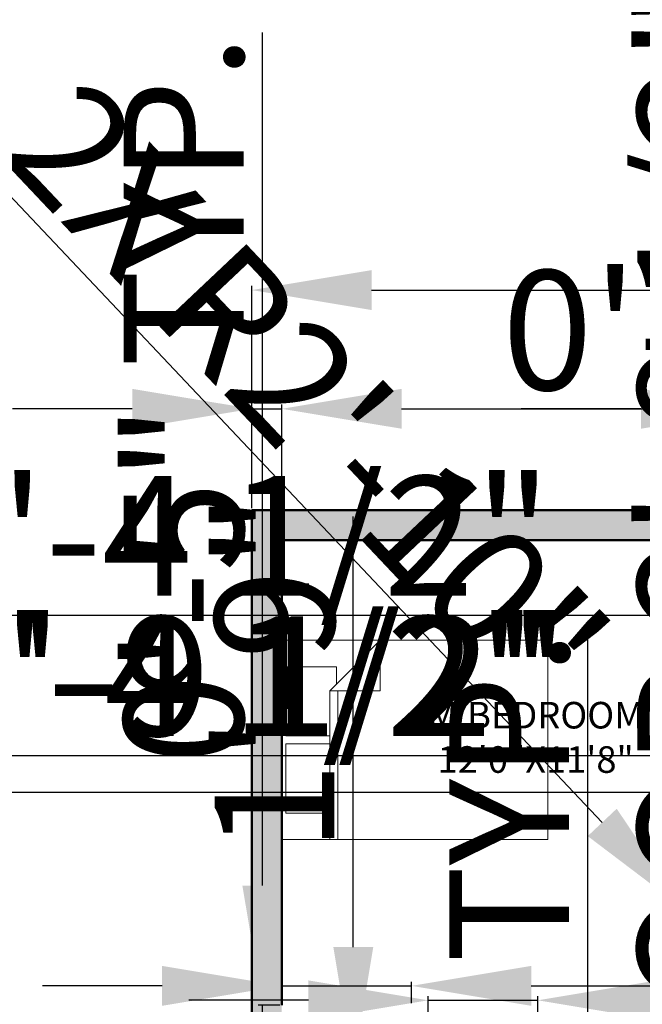
# Model space of a CAD drawing. Units: inches. Extents: x -299 to 1164, y -2 to 940.
# Tile 7 of 11: x 189 to 376, y 490 to 786. Entities that reach past the tile are written whole.
import ezdxf

# ---------------------------------------------------------------- set-up
doc = ezdxf.new("R2010")
doc.units = ezdxf.units.IN
for name, color, linetype, lineweight in [('A-AREA-IDEN', 3, 'Continuous', 25), ('A-FURN', 8, 'Continuous', 18), ('dimensions', 191, 'Continuous', 18), ('outer walls', 7, 'Continuous', 50)]:
    doc.layers.add(name, color=color, linetype=linetype, lineweight=lineweight)
doc.layers.add('A-WALL-PATT', color=240, linetype='Continuous', lineweight=13, true_color=0xed1f24)
doc.styles.get("Standard").update_dxf_attribs({"font": 'arial.ttf'})
doc.dimstyles.new('ISO-25', dxfattribs={"dimtxt": 36, "dimasz": 36, "dimexe": 1.25, "dimexo": 0.625, "dimtad": 1, "dimlunit": 3, "dimtxsty": 'Standard', "dimcen": 2.5, "dimazin": 0, "dimtfac": 1, "dimtmove": 0, "dimatfit": 3, "dimfxl": 1, "dimarcsym": 0})

# ---------------------------------------------------------------- blocks, each defined once
blk = doc.blocks.new('Bed - Queen')
for p, q in [((0, -80.00003), (0, 0)), ((0, 0), (59.99999, 0)), ((59.99999, 0), (59.99999, -80.00003)), ((7.99999, -1.2), (28.79998, -1.2)), ((7.99999, -14.4), (7.99999, -1.2)), ((28.79998, -1.2), (28.79998, -14.4)), ((31.19999, -1.2), (51.99999, -1.2)), ((31.19999, -14.4), (31.19999, -1.2)), ((51.99999, -1.2), (51.99999, -16.4)), ((0, -14.4), (44.8, -14.4)), ((59.99999, -29.6), (44.8, -14.4)), ((44.8, -14.4), (44.8, -29.6)), ((44.8, -16.8), (0, -16.8)), ((51.99999, -16.4), (46.79936, -16.4)), ((44.8, -29.6), (59.99999, -29.6)), ((59.99999, -80.00003), (0, -80.00003))]:
    blk.add_line(p, q)
blk = doc.blocks.new('*D13')
at = {"layer": 'Defpoints', "color": 0, "transparency": 16777216}
for p in [(739.07, 704.71), (259.07, 638.49), (739.07, 638.49)]:
    blk.add_point(p, dxfattribs=at)
at = {"layer": 'dimensions', "color": 0, "lineweight": -2, "transparency": 16777216}
for p, q in [((259.07, 639.11), (259.07, 705.96)), ((739.07, 639.11), (739.07, 705.96)), ((295.07, 704.71), (703.07, 704.71))]:
    blk.add_line(p, q, dxfattribs=at)
at = {"layer": 'dimensions', "color": 0, "transparency": 16777216}
for points in [[(295.07, 710.71), (295.07, 698.71), (259.07, 704.71)], [(703.07, 710.71), (703.07, 698.71), (739.07, 704.71)]]:
    blk.add_solid(points, dxfattribs=at)
at = {"layer": 'dimensions', "color": 0, "transparency": 16777216, "insert": (499.07, 723.71), "char_height": 36, "attachment_point": 5}
blk.add_mtext("40'", dxfattribs=at)
blk = doc.blocks.new('*D26')
at = {"layer": 'Defpoints', "color": 0, "transparency": 16777216}
for p in [(415.32, 606.83), (415.32, 597.1), (443.65, 597.1)]:
    blk.add_point(p, dxfattribs=at)
at = {"layer": 'dimensions', "color": 0, "lineweight": -2, "transparency": 16777216}
for p, q in [((415.32, 597.72), (415.32, 608.08)), ((443.65, 597.72), (443.65, 608.08)), ((379.32, 606.83), (161.88, 606.83)), ((443.65, 606.83), (415.32, 606.83)), ((479.65, 606.83), (515.65, 606.83))]:
    blk.add_line(p, q, dxfattribs=at)
at = {"layer": 'dimensions', "color": 0, "transparency": 16777216}
for points in [[(379.32, 612.83), (379.32, 600.83), (415.32, 606.83)], [(479.65, 612.83), (479.65, 600.83), (443.65, 606.83)]]:
    blk.add_solid(points, dxfattribs=at)
at = {"layer": 'dimensions', "color": 0, "transparency": 16777216, "insert": (252.6, 626.07), "char_height": 36, "attachment_point": 5}
blk.add_mtext('2\'-4 1/2"', dxfattribs=at)
blk = doc.blocks.new('*D27')
at = {"layer": 'Defpoints', "color": 0, "transparency": 16777216}
for p in [(412.07, 375.49), (416.95, 375.49), (412.07, 342.99)]:
    blk.add_point(p, dxfattribs=at)
at = {"layer": 'dimensions', "color": 0, "lineweight": -2, "transparency": 16777216}
for p, q in [((416.95, 411.49), (416.95, 915.12)), ((412.7, 375.49), (418.2, 375.49)), ((416.95, 342.99), (416.95, 375.49)), ((412.7, 342.99), (418.2, 342.99)), ((416.95, 306.99), (416.95, 270.99))]:
    blk.add_line(p, q, dxfattribs=at)
at = {"layer": 'dimensions', "color": 0, "transparency": 16777216}
for points in [[(410.95, 411.49), (422.95, 411.49), (416.95, 375.49)], [(410.95, 306.99), (422.95, 306.99), (416.95, 342.99)]]:
    blk.add_solid(points, dxfattribs=at)
at = {"layer": 'dimensions', "color": 0, "transparency": 16777216, "insert": (397.69, 681.3), "char_height": 36, "attachment_point": 5, "rotation": 90}
blk.add_mtext('DOOR 2\'-8 1/2" TYP.', dxfattribs=at)
blk = doc.blocks.new('*D32')
at = {"layer": 'Defpoints', "color": 0, "transparency": 16777216}
for p in [(348.07, 310.2), (360.07, 310.2), (348.07, 250.2)]:
    blk.add_point(p, dxfattribs=at)
at = {"layer": 'dimensions', "color": 0, "lineweight": -2, "transparency": 16777216}
for p, q in [((360.07, 346.2), (360.07, 602.89)), ((348.7, 310.2), (361.32, 310.2)), ((360.07, 250.2), (360.07, 310.2)), ((348.7, 250.2), (361.32, 250.2)), ((360.07, 214.2), (360.07, 178.2))]:
    blk.add_line(p, q, dxfattribs=at)
at = {"layer": 'dimensions', "color": 0, "transparency": 16777216}
for points in [[(354.07, 346.2), (366.07, 346.2), (360.07, 310.2)], [(354.07, 214.2), (366.07, 214.2), (360.07, 250.2)]]:
    blk.add_solid(points, dxfattribs=at)
at = {"layer": 'dimensions', "color": 0, "transparency": 16777216, "insert": (341.07, 492.55), "char_height": 36, "attachment_point": 5, "rotation": 90}
blk.add_mtext('5\'-0" TYP.', dxfattribs=at)
blk = doc.blocks.new('*D34')
at = {"layer": 'Defpoints', "color": 0, "transparency": 16777216}
for p in [(443.84, 222.49), (447.44, 222.49), (443.84, 213.49)]:
    blk.add_point(p, dxfattribs=at)
at = {"layer": 'dimensions', "color": 0, "lineweight": -2, "transparency": 16777216}
for p, q in [((447.44, 258.49), (447.44, 515.18)), ((444.47, 222.49), (448.69, 222.49)), ((447.44, 213.49), (447.44, 222.49)), ((444.47, 213.49), (448.69, 213.49)), ((447.44, 177.49), (447.44, 141.49))]:
    blk.add_line(p, q, dxfattribs=at)
at = {"layer": 'dimensions', "color": 0, "transparency": 16777216}
for points in [[(441.44, 258.49), (453.44, 258.49), (447.44, 222.49)], [(441.44, 177.49), (453.44, 177.49), (447.44, 213.49)]]:
    blk.add_solid(points, dxfattribs=at)
at = {"layer": 'dimensions', "color": 0, "transparency": 16777216, "insert": (428.44, 404.83), "char_height": 36, "attachment_point": 5, "rotation": 90}
blk.add_mtext('0\'-9" TYP.', dxfattribs=at)
blk = doc.blocks.new('*D35')
at = {"layer": 'Defpoints', "color": 0, "transparency": 16777216}
for p in [(307.07, 495.34), (268.07, 489.49), (307.07, 489.49)]:
    blk.add_point(p, dxfattribs=at)
at = {"layer": 'dimensions', "color": 0, "lineweight": -2, "transparency": 16777216}
for p, q in [((232.07, 495.34), (196.07, 495.34)), ((268.07, 490.11), (268.07, 496.59)), ((268.07, 495.34), (307.07, 495.34)), ((307.07, 490.11), (307.07, 496.59)), ((343.07, 495.34), (749.73, 495.34))]:
    blk.add_line(p, q, dxfattribs=at)
at = {"layer": 'dimensions', "color": 0, "transparency": 16777216}
for points in [[(232.07, 501.34), (232.07, 489.34), (268.07, 495.34)], [(343.07, 501.34), (343.07, 489.34), (307.07, 495.34)]]:
    blk.add_solid(points, dxfattribs=at)
at = {"layer": 'dimensions', "color": 0, "transparency": 16777216, "insert": (564.4, 514.36), "char_height": 36, "attachment_point": 5}
blk.add_mtext('VENT 3\'-3" TYP.', dxfattribs=at)
blk = doc.blocks.new('*D36')
at = {"layer": 'Defpoints', "color": 0, "transparency": 16777216}
for p in [(262.22, 489.49), (268.07, 489.49), (268.07, 484.49)]:
    blk.add_point(p, dxfattribs=at)
at = {"layer": 'dimensions', "color": 0, "lineweight": -2, "transparency": 16777216}
for p, q in [((262.22, 525.49), (262.22, 782.18)), ((267.45, 489.49), (260.97, 489.49)), ((262.22, 484.49), (262.22, 489.49)), ((267.45, 484.49), (260.97, 484.49)), ((262.22, 448.49), (262.22, 412.49))]:
    blk.add_line(p, q, dxfattribs=at)
at = {"layer": 'dimensions', "color": 0, "transparency": 16777216}
for points in [[(256.22, 525.49), (268.22, 525.49), (262.22, 489.49)], [(256.22, 448.49), (268.22, 448.49), (262.22, 484.49)]]:
    blk.add_solid(points, dxfattribs=at)
at = {"layer": 'dimensions', "color": 0, "transparency": 16777216, "insert": (243.22, 671.83), "char_height": 36, "attachment_point": 5, "rotation": 90}
blk.add_mtext('0\'-5" TYP.', dxfattribs=at)
blk = doc.blocks.new('*D43')
at = {"layer": 'Defpoints', "color": 0, "transparency": 16777216}
for p in [(268.07, 668.99), (259.07, 638.49), (268.07, 629.49)]:
    blk.add_point(p, dxfattribs=at)
at = {"layer": 'dimensions', "color": 0, "lineweight": -2, "transparency": 16777216}
for p, q in [((259.07, 639.11), (259.07, 670.24)), ((268.07, 630.11), (268.07, 670.24)), ((223.07, 668.99), (187.07, 668.99)), ((259.07, 668.99), (268.07, 668.99)), ((304.07, 668.99), (437.02, 668.99))]:
    blk.add_line(p, q, dxfattribs=at)
at = {"layer": 'dimensions', "color": 0, "transparency": 16777216}
for points in [[(223.07, 674.99), (223.07, 662.99), (259.07, 668.99)], [(304.07, 674.99), (304.07, 662.99), (268.07, 668.99)]]:
    blk.add_solid(points, dxfattribs=at)
at = {"layer": 'dimensions', "color": 0, "transparency": 16777216, "insert": (388.54, 687.99), "char_height": 36, "attachment_point": 5}
blk.add_mtext('0\'-9"', dxfattribs=at)
blk = doc.blocks.new('*D44')
at = {"layer": 'Defpoints', "color": 0, "transparency": 16777216}
for p in [(417.07, 668.99), (412.07, 629.49), (417.07, 629.49)]:
    blk.add_point(p, dxfattribs=at)
at = {"layer": 'dimensions', "color": 0, "lineweight": -2, "transparency": 16777216}
for p, q in [((412.07, 630.11), (412.07, 670.24)), ((417.07, 630.11), (417.07, 670.24)), ((376.07, 668.99), (340.07, 668.99)), ((412.07, 668.99), (417.07, 668.99)), ((453.07, 668.99), (586.02, 668.99))]:
    blk.add_line(p, q, dxfattribs=at)
at = {"layer": 'dimensions', "color": 0, "transparency": 16777216}
for points in [[(376.07, 674.99), (376.07, 662.99), (412.07, 668.99)], [(453.07, 674.99), (453.07, 662.99), (417.07, 668.99)]]:
    blk.add_solid(points, dxfattribs=at)
at = {"layer": 'dimensions', "color": 0, "transparency": 16777216, "insert": (537.54, 687.99), "char_height": 36, "attachment_point": 5}
blk.add_mtext('0\'-5"', dxfattribs=at)
blk = doc.blocks.new('*D53')
at = {"layer": 'Defpoints', "color": 0, "transparency": 16777216}
for p in [(177.57, 553.49), (586.07, 553.49), (586.07, 481.49)]:
    blk.add_point(p, dxfattribs=at)
at = {"layer": 'dimensions', "color": 0, "lineweight": -2, "transparency": 16777216}
for p, q in [((177.57, 589.49), (177.57, 722.63)), ((585.45, 553.49), (176.32, 553.49)), ((177.57, 481.49), (177.57, 553.49)), ((585.45, 481.49), (176.32, 481.49)), ((177.57, 445.49), (177.57, 409.49))]:
    blk.add_line(p, q, dxfattribs=at)
at = {"layer": 'dimensions', "color": 0, "transparency": 16777216}
for points in [[(171.57, 589.49), (183.57, 589.49), (177.57, 553.49)], [(171.57, 445.49), (183.57, 445.49), (177.57, 481.49)]]:
    blk.add_solid(points, dxfattribs=at)
at = {"layer": 'dimensions', "color": 0, "transparency": 16777216, "insert": (158.57, 674.06), "char_height": 36, "attachment_point": 5, "rotation": 90}
blk.add_mtext('6\'-0"', dxfattribs=at)
blk = doc.blocks.new('*D54')
at = {"layer": 'Defpoints', "color": 0, "transparency": 16777216}
for p in [(345.07, 490.99), (312.07, 460.49), (345.07, 460.49)]:
    blk.add_point(p, dxfattribs=at)
at = {"layer": 'dimensions', "color": 0, "lineweight": -2, "transparency": 16777216}
for p, q in [((312.07, 461.11), (312.07, 492.24)), ((345.07, 461.11), (345.07, 492.24)), ((276.07, 490.99), (240.07, 490.99)), ((312.07, 490.99), (345.07, 490.99)), ((381.07, 490.99), (514.63, 490.99))]:
    blk.add_line(p, q, dxfattribs=at)
at = {"layer": 'dimensions', "color": 0, "transparency": 16777216}
for points in [[(276.07, 496.99), (276.07, 484.99), (312.07, 490.99)], [(381.07, 496.99), (381.07, 484.99), (345.07, 490.99)]]:
    blk.add_solid(points, dxfattribs=at)
at = {"layer": 'dimensions', "color": 0, "transparency": 16777216, "insert": (465.85, 509.99), "char_height": 36, "attachment_point": 5}
blk.add_mtext('2\'-9"', dxfattribs=at)
blk = doc.blocks.new('*D55')
at = {"layer": 'Defpoints', "color": 0, "transparency": 16777216}
for p in [(289.57, 470.99), (320.07, 470.99), (320.07, 449.99)]:
    blk.add_point(p, dxfattribs=at)
at = {"layer": 'dimensions', "color": 0, "lineweight": -2, "transparency": 16777216}
for p, q in [((289.57, 506.99), (289.57, 636.55)), ((319.45, 470.99), (288.32, 470.99)), ((289.57, 449.99), (289.57, 470.99)), ((319.45, 449.99), (288.32, 449.99)), ((289.57, 413.99), (289.57, 377.99))]:
    blk.add_line(p, q, dxfattribs=at)
at = {"layer": 'dimensions', "color": 0, "transparency": 16777216}
for points in [[(283.57, 506.99), (295.57, 506.99), (289.57, 470.99)], [(283.57, 413.99), (295.57, 413.99), (289.57, 449.99)]]:
    blk.add_solid(points, dxfattribs=at)
at = {"layer": 'dimensions', "color": 0, "transparency": 16777216, "insert": (270.57, 589.77), "char_height": 36, "attachment_point": 5, "rotation": 90}
blk.add_mtext('1\'-9"', dxfattribs=at)
blk = doc.blocks.new('*D61')
at = {"layer": 'Defpoints', "color": 0, "transparency": 16777216}
for p in [(389.15, 518.35), (412.32, 493.81)]:
    blk.add_point(p, dxfattribs=at)
at = {"layer": 'dimensions', "color": 0, "lineweight": -2, "transparency": 16777216}
for p, q in [((176.74, 743.24), (364.43, 544.52)), ((412.32, 493.81), (389.15, 518.35))]:
    blk.add_line(p, q, dxfattribs=at)
at = {"layer": 'dimensions', "color": 0, "transparency": 16777216}
blk.add_solid([(368.79, 548.64), (360.07, 540.4), (389.15, 518.35)], dxfattribs=at)
at = {"layer": 'dimensions', "color": 0, "transparency": 16777216, "insert": (272.04, 670.02), "char_height": 36, "attachment_point": 5, "rotation": 313.3644}
blk.add_mtext('2X R2\'-10"', dxfattribs=at)
blk = doc.blocks.new('*D68')
at = {"layer": 'Defpoints', "color": 0, "transparency": 16777216}
for p in [(422.02, 564.66), (515.63, 564.66)]:
    blk.add_point(p, dxfattribs=at)
at = {"layer": 'dimensions', "color": 0, "lineweight": -2, "transparency": 16777216}
for p, q in [((134.73, 564.66), (386.02, 564.66)), ((515.63, 564.66), (422.02, 564.66))]:
    blk.add_line(p, q, dxfattribs=at)
at = {"layer": 'dimensions', "color": 0, "transparency": 16777216}
blk.add_solid([(386.02, 570.66), (386.02, 558.66), (422.02, 564.66)], dxfattribs=at)
at = {"layer": 'dimensions', "color": 0, "transparency": 16777216, "insert": (242.37, 583.9), "char_height": 36, "attachment_point": 5, "rotation": 359.9997}
blk.add_mtext('R7\'-9 1/2"', dxfattribs=at)
blk = doc.blocks.new('*D70')
at = {"layer": 'Defpoints', "color": 0, "transparency": 16777216}
for p in [(417.38, 564.66), (505.63, 564.66)]:
    blk.add_point(p, dxfattribs=at)
at = {"layer": 'dimensions', "color": 0, "lineweight": -2, "transparency": 16777216}
for p, q in [((130.1, 564.66), (381.38, 564.66)), ((505.63, 564.66), (417.38, 564.66))]:
    blk.add_line(p, q, dxfattribs=at)
at = {"layer": 'dimensions', "color": 0, "transparency": 16777216}
blk.add_solid([(381.38, 570.66), (381.38, 558.66), (417.38, 564.66)], dxfattribs=at)
at = {"layer": 'dimensions', "color": 0, "transparency": 16777216, "insert": (237.74, 583.9), "char_height": 36, "attachment_point": 5, "rotation": 359.9997}
blk.add_mtext('R7\'-4 1/2"', dxfattribs=at)

msp = doc.modelspace()

# ---------------------------------------------------------------- hatches: boundary and pattern name
at = {"layer": 'A-WALL-PATT'}
h = msp.add_hatch(color=256, dxfattribs=at)
h.dxf.hatch_style = 1
h.paths.add_polyline_path([(312.071, 460.489), (307.071, 460.489), (307.071, 432.489), (307.071, 427.489), (372.071, 427.489), (372.071, 375.489), (372.071, 370.489), (380.071, 370.489, -0.0217424), (380.071, 372.989), (380.071, 375.489), (377.071, 375.489), (377.071, 427.489), (417.071, 427.489), (417.071, 489.489), (412.071, 489.489), (412.071, 484.489), (412.071, 432.489), (312.071, 432.489)], flags=17)
h.paths.add_polyline_path([(340.071, 372.989, -0.0217424), (340.071, 375.489), (268.071, 375.489), (268.071, 427.489), (268.071, 432.489), (268.071, 484.489), (268.071, 489.489), (268.071, 629.489), (412.071, 629.489), (412.071, 527.563, -0.0185322), (414.571, 527.489), (417.071, 527.489), (417.071, 629.489), (581.071, 629.489), (581.071, 553.489), (586.071, 553.489), (586.071, 629.489), (730.071, 629.489), (730.071, 405.489), (713.071, 405.489), (713.071, 396.489), (739.071, 396.489), (739.071, 638.489), (259.071, 638.489), (259.071, 183.489), (304.071, 183.489), (304.071, 192.489), (268.071, 192.489), (268.071, 370.489), (340.071, 370.489)])
h.paths.add_polyline_path([(417.071, 188.489), (417.071, 213.489), (461.071, 213.489), (461.071, 188.489)], flags=16)
h.paths.add_polyline_path([(586.071, 313.578), (577.071, 313.578), (577.071, 311.489), (575.54, 311.489), (575.54, 302.489), (586.071, 302.489)], flags=16)
h.paths.add_polyline_path([(586.071, 405.489), (586.071, 481.489), (581.071, 481.489), (581.071, 432.489), (499.071, 432.489), (499.071, 427.489), (577.071, 427.489), (577.071, 385.578), (586.071, 385.578), (586.071, 396.489)], flags=17)
h.paths.add_polyline_path([(641.071, 405.489), (624.071, 405.489, -0.0333689), (624.071, 400.989), (624.071, 396.489), (641.071, 396.489)], flags=17)
h.paths.add_polyline_path([(491.866, 222.489), (491.866, 213.489), (586.071, 213.489), (586.071, 222.489)])
edge = h.paths.add_edge_path()
edge.add_line((467.866, 213.489), (467.866, 222.489))
edge.add_line((467.866, 222.489), (466.071, 222.489))
edge.add_line((466.071, 222.489), (466.071, 302.489))
edge.add_line((466.071, 302.489), (527.54, 302.489))
edge.add_line((527.54, 302.489), (527.54, 311.489))
edge.add_line((527.54, 311.489), (449.071, 311.489))
edge.add_line((449.071, 311.489), (449.071, 308.989))
edge.add_arc((420.339, 307.739), 28.759, -2.4911, 2.4911, ccw=False)
edge.add_line((449.071, 306.489), (461.071, 306.489))
edge.add_line((461.071, 306.489), (461.071, 222.489))
edge.add_line((461.071, 222.489), (443.844, 222.489))
edge.add_line((443.844, 222.489), (443.844, 213.489))
edge.add_line((443.844, 213.489), (419.844, 213.489))
edge.add_line((419.844, 213.489), (419.844, 222.489))
edge.add_line((419.844, 222.489), (417.071, 222.489))
edge.add_line((417.071, 222.489), (417.071, 306.489))
edge.add_line((417.071, 306.489), (417.071, 311.489))
edge.add_line((417.071, 311.489), (417.071, 375.489))
edge.add_line((417.071, 375.489), (412.071, 375.489))
edge.add_line((412.071, 375.489), (412.071, 370.489))
edge.add_line((412.071, 370.489), (412.071, 192.489))
edge.add_line((412.071, 192.489), (376.071, 192.489))
edge.add_line((376.071, 192.489), (376.071, 183.489))
edge.add_line((376.071, 183.489), (412.071, 183.489))
edge.add_line((412.071, 183.489), (466.071, 183.489))
edge.add_line((466.071, 183.489), (466.071, 213.489))
edge.add_line((466.071, 213.489), (467.866, 213.489))

# ---------------------------------------------------------------- linework, layer by layer
at = {"layer": 'outer walls'}
for p, q in [((739.071, 638.489), (259.071, 638.489)), ((259.071, 638.489), (259.071, 158.489)), ((268.071, 629.489), (268.071, 489.489)), ((412.071, 629.489), (268.071, 629.489))]:
    msp.add_line(p, q, dxfattribs=at)

# ---------------------------------------------------------------- block references
at = {"layer": 'A-FURN', "rotation": 90}
msp.add_blockref('Bed - Queen', (268.071, 539.336), dxfattribs=at)

# ---------------------------------------------------------------- texts
at = {"layer": 'A-AREA-IDEN', "insert": (309.479, 580.785), "char_height": 8, "attachment_point": 1}
msp.add_mtext_dynamic_manual_height_columns('\\pxqc,t15;M.BEDROOM\\P12\'0"X11\'8"', width=69.83809, gutter_width=12.5, heights=[0], dxfattribs=at)

# ---------------------------------------------------------------- dimensions: what is measured, and where the dimension line sits
at = {"layer": 'dimensions'}
for base, p1, p2, text, picture, middle in [((416.946, 375.489), (412.071, 342.989), (412.071, 375.489), 'DOOR <> TYP.', '*D27', (397.695, 681.304)), ((262.221, 489.489), (268.071, 484.489), (268.071, 489.489), '<> TYP.', '*D36', (243.215, 671.833)), ((360.071, 310.202), (348.071, 250.202), (348.071, 310.202), '<> TYP.', '*D32', (341.065, 492.546)), ((447.444, 222.489), (443.844, 213.489), (443.844, 222.489), '<> TYP.', '*D34', (428.438, 404.833))]:
    dim = msp.add_linear_dim(base=base, p1=p1, p2=p2, angle=90, text=text, dimstyle='ISO-25', override={"dimdec": 1, "dimlfac": 1, "dimrnd": 0, "dimzin": 1, "dimdsep": 46, "dimlunit": 4, "dimfrac": 2}, dxfattribs=at)
    dim.commit()
    dim.dimension.update_dxf_attribs({"geometry": picture, "text_midpoint": middle})
dim = msp.add_radius_dim(center=(412.321, 493.813), mpoint=(389.146, 518.35), text='2X <>', dimstyle='ISO-25', override={"dimdec": 1, "dimlfac": 1, "dimrnd": 0, "dimzin": 1, "dimdsep": 46, "dimlunit": 4, "dimfrac": 2}, dxfattribs=at)
dim.commit()
dim.dimension.update_dxf_attribs({"geometry": '*D61', "text_midpoint": (272.043, 670.016)})
for base, p1, p2, override, picture, middle in [((739.071, 704.705), (259.071, 638.489), (739.071, 638.489), {"dimclrd": 0, "dimclre": 0, "dimclrt": 0}, '*D13', (499.071, 723.711)), ((268.071, 668.989), (259.071, 638.489), (268.071, 629.489), {"dimdec": 1, "dimlfac": 1, "dimrnd": 0, "dimzin": 1, "dimdsep": 46, "dimlunit": 4, "dimfrac": 2}, '*D43', (388.545, 687.995)), ((417.071, 668.989), (412.071, 629.489), (417.071, 629.489), {"dimdec": 1, "dimlfac": 1, "dimrnd": 0, "dimzin": 1, "dimdsep": 46, "dimlunit": 4, "dimfrac": 2}, '*D44', (537.545, 687.995))]:
    dim = msp.add_linear_dim(base=base, p1=p1, p2=p2, dimstyle='ISO-25', override=override, dxfattribs=at)
    dim.commit()
    dim.dimension.update_dxf_attribs({"geometry": picture, "text_midpoint": middle})
for base, p1, p2, angle, picture, middle in [((177.571, 553.489), (586.071, 481.489), (586.071, 553.489), 90, '*D53', (158.565, 674.061)), ((415.323, 606.831), (443.646, 597.099), (415.323, 597.099), 180, '*D26', (252.6, 626.07)), ((289.571, 470.989), (320.071, 449.989), (320.071, 470.989), 90, '*D55', (270.565, 589.768)), ((345.071, 490.989), (312.071, 460.489), (345.071, 460.489), 0.00004, '*D54', (465.852, 509.995))]:
    dim = msp.add_linear_dim(base=base, p1=p1, p2=p2, angle=angle, dimstyle='ISO-25', override={"dimdec": 1, "dimlfac": 1, "dimrnd": 0, "dimzin": 1, "dimdsep": 46, "dimlunit": 4, "dimfrac": 2}, dxfattribs=at)
    dim.commit()
    dim.dimension.update_dxf_attribs({"geometry": picture, "text_midpoint": middle})
for center, mpoint, picture, middle in [((505.6333, 564.6566), (417.383, 564.657), '*D70', (237.7404, 583.8968)), ((515.634, 564.657), (422.018, 564.657), '*D68', (242.375, 583.897))]:
    dim = msp.add_radius_dim(center=center, mpoint=mpoint, dimstyle='ISO-25', override={"dimdec": 1, "dimlfac": 1, "dimrnd": 0, "dimzin": 1, "dimdsep": 46, "dimlunit": 4, "dimfrac": 2}, dxfattribs=at)
    dim.commit()
    dim.dimension.update_dxf_attribs({"geometry": picture, "text_midpoint": middle})
dim = msp.add_linear_dim(base=(307.071, 495.339), p1=(268.071, 489.489), p2=(307.071, 489.489), text='VENT <> TYP.', dimstyle='ISO-25', override={"dimdec": 1, "dimlfac": 1, "dimrnd": 0, "dimzin": 1, "dimdsep": 46, "dimlunit": 4, "dimfrac": 2}, dxfattribs=at)
dim.commit()
dim.dimension.update_dxf_attribs({"geometry": '*D35', "text_midpoint": (564.399, 514.357)})

doc.saveas('drawing.dxf')
